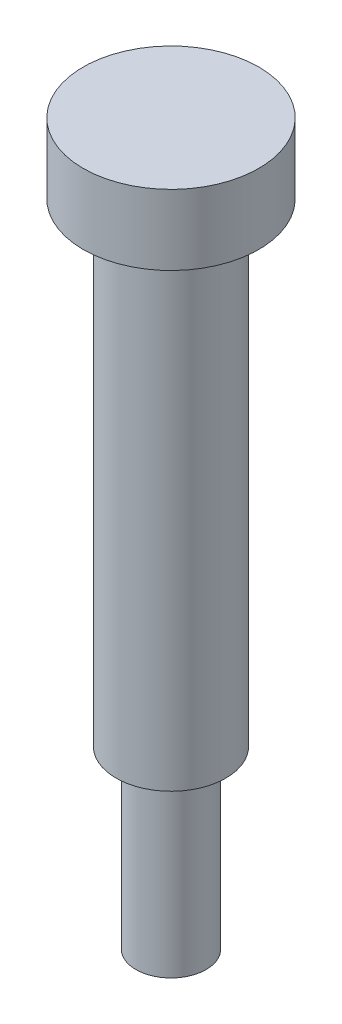
from build123d import *


with BuildPart() as part:
    # Screw Profile Sketch → Screw Body Revolve (revolve)
    with BuildSketch(Plane.XY, mode=Mode.PRIVATE) as screw_body_revolve_sk:
        Polygon((0, 0), (-2, 0), (-2, 10), (-3.125, 10), (-3.125, 37), (-5, 37), (-5, 41), (0, 41), align=None)
    revolve(screw_body_revolve_sk.sketch.rotate(Axis((0, 0, 0), (0, 1, 0)), 270), axis=Axis((0, 0, 0), (0, 1, 0)))


solid = part.part
